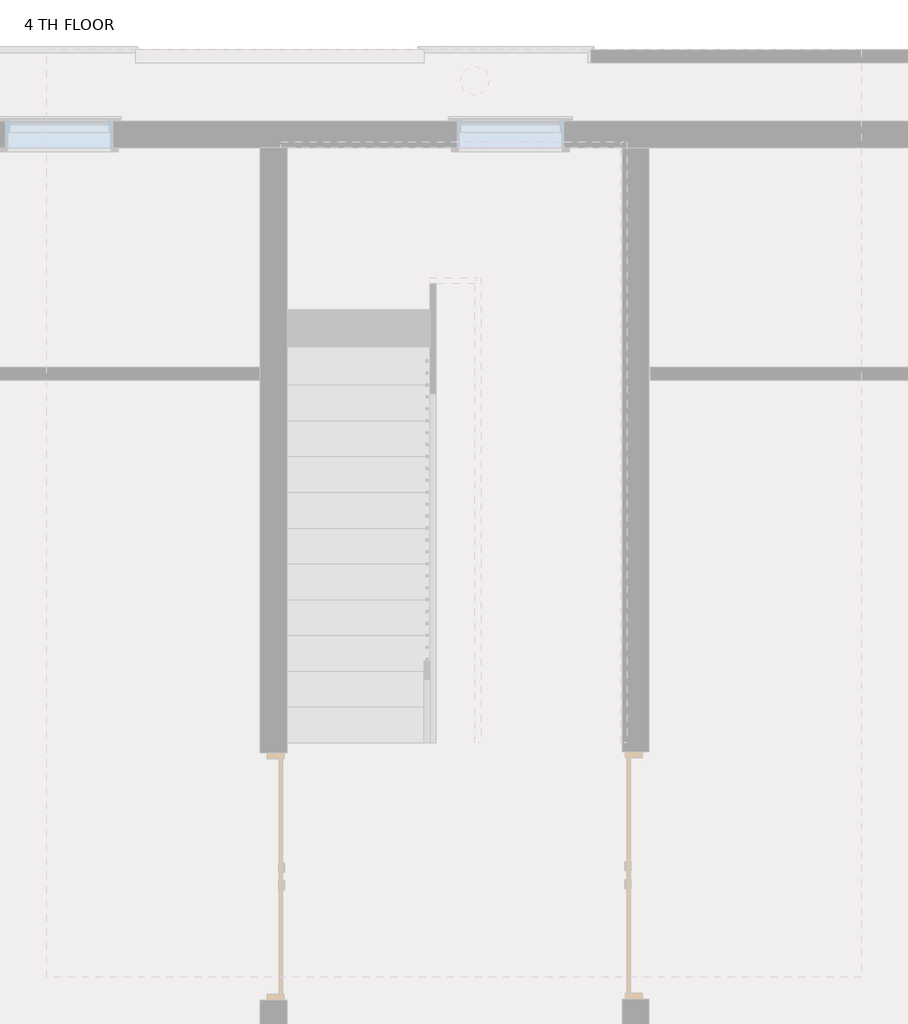
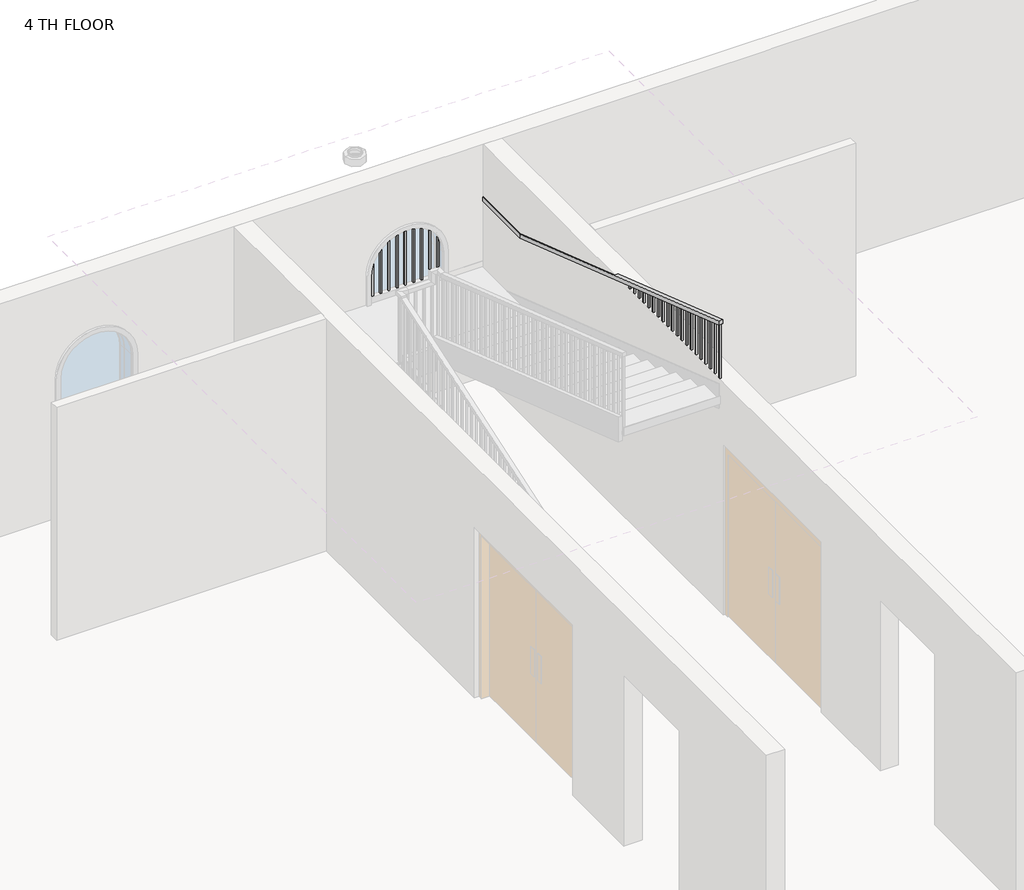
# One storey, part 5 of 7: 1 railing.
"""IFC4 building model written with IfcOpenShell, lengths in millimetres."""

from ifc_helpers import new_model, si_unit, frame, origin, place, context, project, spatial, polyline, outline, extrude, faceted_brep, element, save

model = new_model("IFC4")

# Units and contexts
model_context = context("Model", 3, world=origin())
ifc_project = project(units=[si_unit("LENGTHUNIT", "METRE", prefix="MILLI")], contexts=[model_context])

# Site, building, storey
site = spatial("IfcSite", under=ifc_project)
building = spatial("IfcBuilding", under=site)
storey = spatial("IfcBuildingStorey", under=building, Name="4 TH FLOOR", Elevation=12801.6)

# Railing
placement = place(None, origin())
element("IfcRailing", 1, ObjectType="Handrail - Rectangular", at=placement, inside=storey, context=model_context, shape_type="SolidModel", body=[
    faceted_brep([(-1899.5987998, 2564.5067329, 13819.4142857), (-1899.5987998, 2564.5067329, 13765.7699957), (-1848.7987998, 2564.5067329, 13765.7699957), (-1848.7987998, 2564.5067329, 13819.4142857), (-1899.5987998, 6526.9067329, 15163.8), (-1899.5987998, 6535.2899033, 15113.0), (-1848.7987998, 6535.2899033, 15113.0), (-1848.7987998, 6526.9067329, 15163.8), (-1899.5987998, 7682.6067329, 15113.0), (-1899.5987998, 7682.6067329, 15163.8), (1046.8012002, 7682.6067329, 15163.8), (1046.8012002, 7682.6067329, 15113.0), (-1848.7987998, 7631.8067329, 15113.0), (996.0012002, 7631.8067329, 15113.0), (-1848.7987998, 7631.8067329, 15163.8), (996.0012002, 7631.8067329, 15163.8), (1046.8012002, 6831.7067329, 15163.8), (1046.8012002, 6823.3235624, 15113.0), (996.0012002, 6823.3235624, 15113.0), (996.0012002, 6831.7067329, 15163.8), (1046.8012002, 2564.5067329, 16611.6), (996.0012002, 2564.5067329, 16611.6), (996.0012002, 2564.5067329, 16557.95571), (1046.8012002, 2564.5067329, 16557.95571)], [[[0, 1, 2, 3]], [[1, 0, 4, 5]], [[2, 1, 5, 6]], [[3, 2, 6, 7]], [[0, 3, 7, 4]], [[8, 9, 10, 11]], [[12, 8, 11, 13]], [[14, 12, 13, 15]], [[9, 14, 15, 10]], [[11, 10, 16, 17]], [[13, 11, 17, 18]], [[15, 13, 18, 19]], [[10, 15, 19, 16]], [[5, 4, 9, 8]], [[6, 5, 8, 12]], [[7, 6, 12, 14]], [[4, 7, 14, 9]], [[20, 21, 22, 23]], [[17, 16, 20, 23]], [[18, 17, 23, 22]], [[19, 18, 22, 21]], [[16, 19, 21, 20]]]),
    extrude(outline(polyline([(2586.7317329, 16550.415085), (2586.7317329, 15779.4831452), (2567.6817329, 15785.9465381), (2567.6817329, 16556.8784779), (2586.7317329, 16550.415085)])), frame((1011.8762002, 0.0, 0.0), z_axis=(1.0, 0.0, 0.0), x_axis=(0.0, 1.0, 0.0)), (0.0, 0.0, 1.0), 19.05),
    extrude(outline(polyline([(2688.3317329, 16515.9436565), (2688.3317329, 15745.0117167), (2669.2817329, 15751.4751095), (2669.2817329, 16522.4070493), (2688.3317329, 16515.9436565)])), frame((1011.8762002, 0.0, 0.0), z_axis=(1.0, 0.0, 0.0), x_axis=(0.0, 1.0, 0.0)), (0.0, 0.0, 1.0), 19.05),
    extrude(outline(polyline([(2789.9317329, 16481.4722279), (2789.9317329, 15710.5402881), (2770.8817329, 15717.003681), (2770.8817329, 16487.9356207), (2789.9317329, 16481.4722279)])), frame((1011.8762002, 0.0, 0.0), z_axis=(1.0, 0.0, 0.0), x_axis=(0.0, 1.0, 0.0)), (0.0, 0.0, 1.0), 19.05),
    extrude(outline(polyline([(2891.5317329, 16447.0007993), (2891.5317329, 15676.0688595), (2872.4817329, 15682.5322524), (2872.4817329, 16453.4641922), (2891.5317329, 16447.0007993)])), frame((1011.8762002, 0.0, 0.0), z_axis=(1.0, 0.0, 0.0), x_axis=(0.0, 1.0, 0.0)), (0.0, 0.0, 1.0), 19.05),
    extrude(outline(polyline([(2993.1317329, 16412.5293707), (2993.1317329, 15641.597431), (2974.0817329, 15648.0608238), (2974.0817329, 16418.9927636), (2993.1317329, 16412.5293707)])), frame((1011.8762002, 0.0, 0.0), z_axis=(1.0, 0.0, 0.0), x_axis=(0.0, 1.0, 0.0)), (0.0, 0.0, 1.0), 19.05),
    extrude(outline(polyline([(3094.7317329, 16378.0579422), (3094.7317329, 15607.1260024), (3075.6817329, 15613.5893952), (3075.6817329, 16384.521335), (3094.7317329, 16378.0579422)])), frame((1011.8762002, 0.0, 0.0), z_axis=(1.0, 0.0, 0.0), x_axis=(0.0, 1.0, 0.0)), (0.0, 0.0, 1.0), 19.05),
    extrude(outline(polyline([(3196.3317329, 16343.5865136), (3196.3317329, 15572.6545738), (3177.2817329, 15579.1179667), (3177.2817329, 16350.0499065), (3196.3317329, 16343.5865136)])), frame((1011.8762002, 0.0, 0.0), z_axis=(1.0, 0.0, 0.0), x_axis=(0.0, 1.0, 0.0)), (0.0, 0.0, 1.0), 19.05),
    extrude(outline(polyline([(3297.9317329, 16309.115085), (3297.9317329, 15538.1831452), (3278.8817329, 15544.6465381), (3278.8817329, 16315.5784779), (3297.9317329, 16309.115085)])), frame((1011.8762002, 0.0, 0.0), z_axis=(1.0, 0.0, 0.0), x_axis=(0.0, 1.0, 0.0)), (0.0, 0.0, 1.0), 19.05),
    extrude(outline(polyline([(3399.5317329, 16274.6436565), (3399.5317329, 15503.7117167), (3380.4817329, 15510.1751095), (3380.4817329, 16281.1070493), (3399.5317329, 16274.6436565)])), frame((1011.8762002, 0.0, 0.0), z_axis=(1.0, 0.0, 0.0), x_axis=(0.0, 1.0, 0.0)), (0.0, 0.0, 1.0), 19.05),
    extrude(outline(polyline([(3501.1317329, 16240.1722279), (3501.1317329, 15469.2402881), (3482.0817329, 15475.703681), (3482.0817329, 16246.6356207), (3501.1317329, 16240.1722279)])), frame((1011.8762002, 0.0, 0.0), z_axis=(1.0, 0.0, 0.0), x_axis=(0.0, 1.0, 0.0)), (0.0, 0.0, 1.0), 19.05),
    extrude(outline(polyline([(3602.7317329, 16205.7007993), (3602.7317329, 15434.7688595), (3583.6817329, 15441.2322524), (3583.6817329, 16212.1641922), (3602.7317329, 16205.7007993)])), frame((1011.8762002, 0.0, 0.0), z_axis=(1.0, 0.0, 0.0), x_axis=(0.0, 1.0, 0.0)), (0.0, 0.0, 1.0), 19.05),
    extrude(outline(polyline([(3704.3317329, 16171.2293707), (3704.3317329, 15400.297431), (3685.2817329, 15406.7608238), (3685.2817329, 16177.6927636), (3704.3317329, 16171.2293707)])), frame((1011.8762002, 0.0, 0.0), z_axis=(1.0, 0.0, 0.0), x_axis=(0.0, 1.0, 0.0)), (0.0, 0.0, 1.0), 19.05),
    extrude(outline(polyline([(3805.9317329, 16136.7579422), (3805.9317329, 15365.8260024), (3786.8817329, 15372.2893952), (3786.8817329, 16143.221335), (3805.9317329, 16136.7579422)])), frame((1011.8762002, 0.0, 0.0), z_axis=(1.0, 0.0, 0.0), x_axis=(0.0, 1.0, 0.0)), (0.0, 0.0, 1.0), 19.05),
    extrude(outline(polyline([(3907.5317329, 16102.2865136), (3907.5317329, 15331.3545738), (3888.4817329, 15337.8179667), (3888.4817329, 16108.7499065), (3907.5317329, 16102.2865136)])), frame((1011.8762002, 0.0, 0.0), z_axis=(1.0, 0.0, 0.0), x_axis=(0.0, 1.0, 0.0)), (0.0, 0.0, 1.0), 19.05),
    extrude(outline(polyline([(4009.1317329, 16067.815085), (4009.1317329, 15296.8831452), (3990.0817329, 15303.3465381), (3990.0817329, 16074.2784779), (4009.1317329, 16067.815085)])), frame((1011.8762002, 0.0, 0.0), z_axis=(1.0, 0.0, 0.0), x_axis=(0.0, 1.0, 0.0)), (0.0, 0.0, 1.0), 19.05),
    extrude(outline(polyline([(4110.7317329, 16033.3436565), (4110.7317329, 15262.4117167), (4091.6817329, 15268.8751095), (4091.6817329, 16039.8070493), (4110.7317329, 16033.3436565)])), frame((1011.8762002, 0.0, 0.0), z_axis=(1.0, 0.0, 0.0), x_axis=(0.0, 1.0, 0.0)), (0.0, 0.0, 1.0), 19.05),
    extrude(outline(polyline([(4212.3317329, 15998.8722279), (4212.3317329, 15227.9402881), (4193.2817329, 15234.403681), (4193.2817329, 16005.3356207), (4212.3317329, 15998.8722279)])), frame((1011.8762002, 0.0, 0.0), z_axis=(1.0, 0.0, 0.0), x_axis=(0.0, 1.0, 0.0)), (0.0, 0.0, 1.0), 19.05),
    extrude(outline(polyline([(4313.9317329, 15964.4007993), (4313.9317329, 15193.4688595), (4294.8817329, 15199.9322524), (4294.8817329, 15970.8641922), (4313.9317329, 15964.4007993)])), frame((1011.8762002, 0.0, 0.0), z_axis=(1.0, 0.0, 0.0), x_axis=(0.0, 1.0, 0.0)), (0.0, 0.0, 1.0), 19.05),
    extrude(outline(polyline([(4415.5317329, 15929.9293707), (4415.5317329, 15158.997431), (4396.4817329, 15165.4608238), (4396.4817329, 15936.3927636), (4415.5317329, 15929.9293707)])), frame((1011.8762002, 0.0, 0.0), z_axis=(1.0, 0.0, 0.0), x_axis=(0.0, 1.0, 0.0)), (0.0, 0.0, 1.0), 19.05),
    extrude(outline(polyline([(4517.1317329, 15895.4579422), (4517.1317329, 15124.5260024), (4498.0817329, 15130.9893952), (4498.0817329, 15901.921335), (4517.1317329, 15895.4579422)])), frame((1011.8762002, 0.0, 0.0), z_axis=(1.0, 0.0, 0.0), x_axis=(0.0, 1.0, 0.0)), (0.0, 0.0, 1.0), 19.05),
    extrude(outline(polyline([(4618.7317329, 15860.9865136), (4618.7317329, 15090.0545738), (4599.6817329, 15096.5179667), (4599.6817329, 15867.4499065), (4618.7317329, 15860.9865136)])), frame((1011.8762002, 0.0, 0.0), z_axis=(1.0, 0.0, 0.0), x_axis=(0.0, 1.0, 0.0)), (0.0, 0.0, 1.0), 19.05),
    extrude(outline(polyline([(4720.3317329, 15826.515085), (4720.3317329, 15055.5831452), (4701.2817329, 15062.0465381), (4701.2817329, 15832.9784779), (4720.3317329, 15826.515085)])), frame((1011.8762002, 0.0, 0.0), z_axis=(1.0, 0.0, 0.0), x_axis=(0.0, 1.0, 0.0)), (0.0, 0.0, 1.0), 19.05),
    extrude(outline(polyline([(4821.9317329, 15792.0436565), (4821.9317329, 15021.1117167), (4802.8817329, 15027.5751095), (4802.8817329, 15798.5070493), (4821.9317329, 15792.0436565)])), frame((1011.8762002, 0.0, 0.0), z_axis=(1.0, 0.0, 0.0), x_axis=(0.0, 1.0, 0.0)), (0.0, 0.0, 1.0), 19.05),
    extrude(outline(polyline([(4923.5317329, 15757.5722279), (4923.5317329, 14986.6402881), (4904.4817329, 14993.103681), (4904.4817329, 15764.0356207), (4923.5317329, 15757.5722279)])), frame((1011.8762002, 0.0, 0.0), z_axis=(1.0, 0.0, 0.0), x_axis=(0.0, 1.0, 0.0)), (0.0, 0.0, 1.0), 19.05),
    extrude(outline(polyline([(5025.1317329, 15723.1007993), (5025.1317329, 14952.1688595), (5006.0817329, 14958.6322524), (5006.0817329, 15729.5641922), (5025.1317329, 15723.1007993)])), frame((1011.8762002, 0.0, 0.0), z_axis=(1.0, 0.0, 0.0), x_axis=(0.0, 1.0, 0.0)), (0.0, 0.0, 1.0), 19.05),
    extrude(outline(polyline([(5126.7317329, 15688.6293707), (5126.7317329, 14917.697431), (5107.6817329, 14924.1608238), (5107.6817329, 15695.0927636), (5126.7317329, 15688.6293707)])), frame((1011.8762002, 0.0, 0.0), z_axis=(1.0, 0.0, 0.0), x_axis=(0.0, 1.0, 0.0)), (0.0, 0.0, 1.0), 19.05),
    extrude(outline(polyline([(5228.3317329, 15654.1579422), (5228.3317329, 14883.2260024), (5209.2817329, 14889.6893952), (5209.2817329, 15660.621335), (5228.3317329, 15654.1579422)])), frame((1011.8762002, 0.0, 0.0), z_axis=(1.0, 0.0, 0.0), x_axis=(0.0, 1.0, 0.0)), (0.0, 0.0, 1.0), 19.05),
    extrude(outline(polyline([(5329.9317329, 15619.6865136), (5329.9317329, 14848.7545738), (5310.8817329, 14855.2179667), (5310.8817329, 15626.1499065), (5329.9317329, 15619.6865136)])), frame((1011.8762002, 0.0, 0.0), z_axis=(1.0, 0.0, 0.0), x_axis=(0.0, 1.0, 0.0)), (0.0, 0.0, 1.0), 19.05),
    extrude(outline(polyline([(5431.5317329, 15585.215085), (5431.5317329, 14814.2831452), (5412.4817329, 14820.7465381), (5412.4817329, 15591.6784779), (5431.5317329, 15585.215085)])), frame((1011.8762002, 0.0, 0.0), z_axis=(1.0, 0.0, 0.0), x_axis=(0.0, 1.0, 0.0)), (0.0, 0.0, 1.0), 19.05),
    extrude(outline(polyline([(5533.1317329, 15550.7436565), (5533.1317329, 14779.8117167), (5514.0817329, 14786.2751095), (5514.0817329, 15557.2070493), (5533.1317329, 15550.7436565)])), frame((1011.8762002, 0.0, 0.0), z_axis=(1.0, 0.0, 0.0), x_axis=(0.0, 1.0, 0.0)), (0.0, 0.0, 1.0), 19.05),
    extrude(outline(polyline([(5634.7317329, 15516.2722279), (5634.7317329, 14745.3402881), (5615.6817329, 14751.803681), (5615.6817329, 15522.7356207), (5634.7317329, 15516.2722279)])), frame((1011.8762002, 0.0, 0.0), z_axis=(1.0, 0.0, 0.0), x_axis=(0.0, 1.0, 0.0)), (0.0, 0.0, 1.0), 19.05),
    extrude(outline(polyline([(5736.3317329, 15481.8007993), (5736.3317329, 14710.8688595), (5717.2817329, 14717.3322524), (5717.2817329, 15488.2641922), (5736.3317329, 15481.8007993)])), frame((1011.8762002, 0.0, 0.0), z_axis=(1.0, 0.0, 0.0), x_axis=(0.0, 1.0, 0.0)), (0.0, 0.0, 1.0), 19.05),
    extrude(outline(polyline([(5837.9317329, 15447.3293707), (5837.9317329, 14676.397431), (5818.8817329, 14682.8608238), (5818.8817329, 15453.7927636), (5837.9317329, 15447.3293707)])), frame((1011.8762002, 0.0, 0.0), z_axis=(1.0, 0.0, 0.0), x_axis=(0.0, 1.0, 0.0)), (0.0, 0.0, 1.0), 19.05),
    extrude(outline(polyline([(5939.5317329, 15412.8579422), (5939.5317329, 14641.9260024), (5920.4817329, 14648.3893952), (5920.4817329, 15419.321335), (5939.5317329, 15412.8579422)])), frame((1011.8762002, 0.0, 0.0), z_axis=(1.0, 0.0, 0.0), x_axis=(0.0, 1.0, 0.0)), (0.0, 0.0, 1.0), 19.05),
    extrude(outline(polyline([(6041.1317329, 15378.3865136), (6041.1317329, 14607.4545738), (6022.0817329, 14613.9179667), (6022.0817329, 15384.8499065), (6041.1317329, 15378.3865136)])), frame((1011.8762002, 0.0, 0.0), z_axis=(1.0, 0.0, 0.0), x_axis=(0.0, 1.0, 0.0)), (0.0, 0.0, 1.0), 19.05),
    extrude(outline(polyline([(6142.7317329, 15343.915085), (6142.7317329, 14572.9831452), (6123.6817329, 14579.4465381), (6123.6817329, 15350.3784779), (6142.7317329, 15343.915085)])), frame((1011.8762002, 0.0, 0.0), z_axis=(1.0, 0.0, 0.0), x_axis=(0.0, 1.0, 0.0)), (0.0, 0.0, 1.0), 19.05),
    extrude(outline(polyline([(6244.3317329, 15309.4436565), (6244.3317329, 14538.5117167), (6225.2817329, 14544.9751095), (6225.2817329, 15315.9070493), (6244.3317329, 15309.4436565)])), frame((1011.8762002, 0.0, 0.0), z_axis=(1.0, 0.0, 0.0), x_axis=(0.0, 1.0, 0.0)), (0.0, 0.0, 1.0), 19.05),
    extrude(outline(polyline([(6345.9317329, 15274.9722279), (6345.9317329, 14504.0402881), (6326.8817329, 14510.503681), (6326.8817329, 15281.4356207), (6345.9317329, 15274.9722279)])), frame((1011.8762002, 0.0, 0.0), z_axis=(1.0, 0.0, 0.0), x_axis=(0.0, 1.0, 0.0)), (0.0, 0.0, 1.0), 19.05),
    extrude(outline(polyline([(6447.5317329, 15240.5007993), (6447.5317329, 14469.5688595), (6428.4817329, 14476.0322524), (6428.4817329, 15246.9641922), (6447.5317329, 15240.5007993)])), frame((1011.8762002, 0.0, 0.0), z_axis=(1.0, 0.0, 0.0), x_axis=(0.0, 1.0, 0.0)), (0.0, 0.0, 1.0), 19.05),
    extrude(outline(polyline([(6549.1317329, 15206.0293707), (6549.1317329, 14435.097431), (6530.0817329, 14441.5608238), (6530.0817329, 15212.4927636), (6549.1317329, 15206.0293707)])), frame((1011.8762002, 0.0, 0.0), z_axis=(1.0, 0.0, 0.0), x_axis=(0.0, 1.0, 0.0)), (0.0, 0.0, 1.0), 19.05),
    extrude(outline(polyline([(6650.7317329, 15171.5579422), (6650.7317329, 14400.6260024), (6631.6817329, 14407.0893952), (6631.6817329, 15178.021335), (6650.7317329, 15171.5579422)])), frame((1011.8762002, 0.0, 0.0), z_axis=(1.0, 0.0, 0.0), x_axis=(0.0, 1.0, 0.0)), (0.0, 0.0, 1.0), 19.05),
    extrude(outline(polyline([(6752.3317329, 15137.0865136), (6752.3317329, 14366.1545738), (6733.2817329, 14372.6179667), (6733.2817329, 15143.5499065), (6752.3317329, 15137.0865136)])), frame((1011.8762002, 0.0, 0.0), z_axis=(1.0, 0.0, 0.0), x_axis=(0.0, 1.0, 0.0)), (0.0, 0.0, 1.0), 19.05),
    extrude(outline(polyline([(6853.9317329, 15113.0), (6853.9317329, 14331.6831452), (6834.8817329, 14338.1465381), (6834.8817329, 15113.0), (6853.9317329, 15113.0)])), frame((1011.8762002, 0.0, 0.0), z_axis=(1.0, 0.0, 0.0), x_axis=(0.0, 1.0, 0.0)), (0.0, 0.0, 1.0), 19.05),
    extrude(outline(polyline([(6955.5317329, 15113.0), (6955.5317329, 14297.2117167), (6936.4817329, 14303.6751095), (6936.4817329, 15113.0), (6955.5317329, 15113.0)])), frame((1011.8762002, 0.0, 0.0), z_axis=(1.0, 0.0, 0.0), x_axis=(0.0, 1.0, 0.0)), (0.0, 0.0, 1.0), 19.05),
    extrude(outline(polyline([(7057.1317329, 15113.0), (7057.1317329, 14262.7402881), (7038.0817329, 14269.203681), (7038.0817329, 15113.0), (7057.1317329, 15113.0)])), frame((1011.8762002, 0.0, 0.0), z_axis=(1.0, 0.0, 0.0), x_axis=(0.0, 1.0, 0.0)), (0.0, 0.0, 1.0), 19.05),
    extrude(outline(polyline([(7158.7317329, 15113.0), (7158.7317329, 14228.2688595), (7139.6817329, 14234.7322524), (7139.6817329, 15113.0), (7158.7317329, 15113.0)])), frame((1011.8762002, 0.0, 0.0), z_axis=(1.0, 0.0, 0.0), x_axis=(0.0, 1.0, 0.0)), (0.0, 0.0, 1.0), 19.05),
    extrude(outline(polyline([(7260.3317329, 15113.0), (7260.3317329, 14193.797431), (7241.2817329, 14200.2608238), (7241.2817329, 15113.0), (7260.3317329, 15113.0)])), frame((1011.8762002, 0.0, 0.0), z_axis=(1.0, 0.0, 0.0), x_axis=(0.0, 1.0, 0.0)), (0.0, 0.0, 1.0), 19.05),
    extrude(outline(polyline([(7361.9317329, 15113.0), (7361.9317329, 14159.3260024), (7342.8817329, 14165.7893952), (7342.8817329, 15113.0), (7361.9317329, 15113.0)])), frame((1011.8762002, 0.0, 0.0), z_axis=(1.0, 0.0, 0.0), x_axis=(0.0, 1.0, 0.0)), (0.0, 0.0, 1.0), 19.05),
    extrude(outline(polyline([(7463.5317329, 15113.0), (7463.5317329, 14124.8545738), (7444.4817329, 14131.3179667), (7444.4817329, 15113.0), (7463.5317329, 15113.0)])), frame((1011.8762002, 0.0, 0.0), z_axis=(1.0, 0.0, 0.0), x_axis=(0.0, 1.0, 0.0)), (0.0, 0.0, 1.0), 19.05),
    extrude(outline(polyline([(7565.1317329, 15113.0), (7565.1317329, 14090.3831452), (7546.0817329, 14096.8465381), (7546.0817329, 15113.0), (7565.1317329, 15113.0)])), frame((1011.8762002, 0.0, 0.0), z_axis=(1.0, 0.0, 0.0), x_axis=(0.0, 1.0, 0.0)), (0.0, 0.0, 1.0), 19.05),
    extrude(outline(polyline([(961.0762002, 7666.7317329), (980.1262002, 7666.7317329), (980.1262002, 7647.6817329), (961.0762002, 7647.6817329), (961.0762002, 7666.7317329)])), frame((0.0, 0.0, 14325.6), z_axis=(0.0, 0.0, 1.0), x_axis=(1.0, 0.0, 0.0)), (0.0, 0.0, 1.0), 787.4),
    extrude(outline(polyline([(859.4762002, 7666.7317329), (878.5262002, 7666.7317329), (878.5262002, 7647.6817329), (859.4762002, 7647.6817329), (859.4762002, 7666.7317329)])), frame((0.0, 0.0, 14325.6), z_axis=(0.0, 0.0, 1.0), x_axis=(1.0, 0.0, 0.0)), (0.0, 0.0, 1.0), 787.4),
    extrude(outline(polyline([(757.8762002, 7666.7317329), (776.9262002, 7666.7317329), (776.9262002, 7647.6817329), (757.8762002, 7647.6817329), (757.8762002, 7666.7317329)])), frame((0.0, 0.0, 14325.6), z_axis=(0.0, 0.0, 1.0), x_axis=(1.0, 0.0, 0.0)), (0.0, 0.0, 1.0), 787.4),
    extrude(outline(polyline([(656.2762002, 7666.7317329), (675.3262002, 7666.7317329), (675.3262002, 7647.6817329), (656.2762002, 7647.6817329), (656.2762002, 7666.7317329)])), frame((0.0, 0.0, 14325.6), z_axis=(0.0, 0.0, 1.0), x_axis=(1.0, 0.0, 0.0)), (0.0, 0.0, 1.0), 787.4),
    extrude(outline(polyline([(554.6762002, 7666.7317329), (573.7262002, 7666.7317329), (573.7262002, 7647.6817329), (554.6762002, 7647.6817329), (554.6762002, 7666.7317329)])), frame((0.0, 0.0, 14325.6), z_axis=(0.0, 0.0, 1.0), x_axis=(1.0, 0.0, 0.0)), (0.0, 0.0, 1.0), 787.4),
    extrude(outline(polyline([(453.0762002, 7666.7317329), (472.1262002, 7666.7317329), (472.1262002, 7647.6817329), (453.0762002, 7647.6817329), (453.0762002, 7666.7317329)])), frame((0.0, 0.0, 14325.6), z_axis=(0.0, 0.0, 1.0), x_axis=(1.0, 0.0, 0.0)), (0.0, 0.0, 1.0), 787.4),
    extrude(outline(polyline([(351.4762002, 7666.7317329), (370.5262002, 7666.7317329), (370.5262002, 7647.6817329), (351.4762002, 7647.6817329), (351.4762002, 7666.7317329)])), frame((0.0, 0.0, 14325.6), z_axis=(0.0, 0.0, 1.0), x_axis=(1.0, 0.0, 0.0)), (0.0, 0.0, 1.0), 787.4),
    extrude(outline(polyline([(249.8762002, 7666.7317329), (268.9262002, 7666.7317329), (268.9262002, 7647.6817329), (249.8762002, 7647.6817329), (249.8762002, 7666.7317329)])), frame((0.0, 0.0, 14325.6), z_axis=(0.0, 0.0, 1.0), x_axis=(1.0, 0.0, 0.0)), (0.0, 0.0, 1.0), 787.4),
    extrude(outline(polyline([(148.2762002, 7666.7317329), (167.3262002, 7666.7317329), (167.3262002, 7647.6817329), (148.2762002, 7647.6817329), (148.2762002, 7666.7317329)])), frame((0.0, 0.0, 14325.6), z_axis=(0.0, 0.0, 1.0), x_axis=(1.0, 0.0, 0.0)), (0.0, 0.0, 1.0), 787.4),
    extrude(outline(polyline([(46.6762002, 7666.7317329), (65.7262002, 7666.7317329), (65.7262002, 7647.6817329), (46.6762002, 7647.6817329), (46.6762002, 7666.7317329)])), frame((0.0, 0.0, 14325.6), z_axis=(0.0, 0.0, 1.0), x_axis=(1.0, 0.0, 0.0)), (0.0, 0.0, 1.0), 787.4),
    extrude(outline(polyline([(-54.9237998, 7666.7317329), (-35.8737998, 7666.7317329), (-35.8737998, 7647.6817329), (-54.9237998, 7647.6817329), (-54.9237998, 7666.7317329)])), frame((0.0, 0.0, 14325.6), z_axis=(0.0, 0.0, 1.0), x_axis=(1.0, 0.0, 0.0)), (0.0, 0.0, 1.0), 787.4),
    extrude(outline(polyline([(-156.5237998, 7666.7317329), (-137.4737998, 7666.7317329), (-137.4737998, 7647.6817329), (-156.5237998, 7647.6817329), (-156.5237998, 7666.7317329)])), frame((0.0, 0.0, 14325.6), z_axis=(0.0, 0.0, 1.0), x_axis=(1.0, 0.0, 0.0)), (0.0, 0.0, 1.0), 787.4),
    extrude(outline(polyline([(-258.1237998, 7666.7317329), (-239.0737998, 7666.7317329), (-239.0737998, 7647.6817329), (-258.1237998, 7647.6817329), (-258.1237998, 7666.7317329)])), frame((0.0, 0.0, 14325.6), z_axis=(0.0, 0.0, 1.0), x_axis=(1.0, 0.0, 0.0)), (0.0, 0.0, 1.0), 787.4),
    extrude(outline(polyline([(-359.7237998, 7666.7317329), (-340.6737998, 7666.7317329), (-340.6737998, 7647.6817329), (-359.7237998, 7647.6817329), (-359.7237998, 7666.7317329)])), frame((0.0, 0.0, 14325.6), z_axis=(0.0, 0.0, 1.0), x_axis=(1.0, 0.0, 0.0)), (0.0, 0.0, 1.0), 787.4),
    extrude(outline(polyline([(-461.3237998, 7666.7317329), (-442.2737998, 7666.7317329), (-442.2737998, 7647.6817329), (-461.3237998, 7647.6817329), (-461.3237998, 7666.7317329)])), frame((0.0, 0.0, 14325.6), z_axis=(0.0, 0.0, 1.0), x_axis=(1.0, 0.0, 0.0)), (0.0, 0.0, 1.0), 787.4),
    extrude(outline(polyline([(-562.9237998, 7666.7317329), (-543.8737998, 7666.7317329), (-543.8737998, 7647.6817329), (-562.9237998, 7647.6817329), (-562.9237998, 7666.7317329)])), frame((0.0, 0.0, 14325.6), z_axis=(0.0, 0.0, 1.0), x_axis=(1.0, 0.0, 0.0)), (0.0, 0.0, 1.0), 787.4),
    extrude(outline(polyline([(-664.5237998, 7666.7317329), (-645.4737998, 7666.7317329), (-645.4737998, 7647.6817329), (-664.5237998, 7647.6817329), (-664.5237998, 7666.7317329)])), frame((0.0, 0.0, 14325.6), z_axis=(0.0, 0.0, 1.0), x_axis=(1.0, 0.0, 0.0)), (0.0, 0.0, 1.0), 787.4),
    extrude(outline(polyline([(-766.1237998, 7666.7317329), (-747.0737998, 7666.7317329), (-747.0737998, 7647.6817329), (-766.1237998, 7647.6817329), (-766.1237998, 7666.7317329)])), frame((0.0, 0.0, 14325.6), z_axis=(0.0, 0.0, 1.0), x_axis=(1.0, 0.0, 0.0)), (0.0, 0.0, 1.0), 787.4),
    extrude(outline(polyline([(-867.7237998, 7666.7317329), (-848.6737998, 7666.7317329), (-848.6737998, 7647.6817329), (-867.7237998, 7647.6817329), (-867.7237998, 7666.7317329)])), frame((0.0, 0.0, 14325.6), z_axis=(0.0, 0.0, 1.0), x_axis=(1.0, 0.0, 0.0)), (0.0, 0.0, 1.0), 787.4),
    extrude(outline(polyline([(-969.3237998, 7666.7317329), (-950.2737998, 7666.7317329), (-950.2737998, 7647.6817329), (-969.3237998, 7647.6817329), (-969.3237998, 7666.7317329)])), frame((0.0, 0.0, 14325.6), z_axis=(0.0, 0.0, 1.0), x_axis=(1.0, 0.0, 0.0)), (0.0, 0.0, 1.0), 787.4),
    extrude(outline(polyline([(-1070.9237998, 7666.7317329), (-1051.8737998, 7666.7317329), (-1051.8737998, 7647.6817329), (-1070.9237998, 7647.6817329), (-1070.9237998, 7666.7317329)])), frame((0.0, 0.0, 14325.6), z_axis=(0.0, 0.0, 1.0), x_axis=(1.0, 0.0, 0.0)), (0.0, 0.0, 1.0), 787.4),
    extrude(outline(polyline([(-1172.5237998, 7666.7317329), (-1153.4737998, 7666.7317329), (-1153.4737998, 7647.6817329), (-1172.5237998, 7647.6817329), (-1172.5237998, 7666.7317329)])), frame((0.0, 0.0, 14325.6), z_axis=(0.0, 0.0, 1.0), x_axis=(1.0, 0.0, 0.0)), (0.0, 0.0, 1.0), 787.4),
    extrude(outline(polyline([(-1274.1237998, 7666.7317329), (-1255.0737998, 7666.7317329), (-1255.0737998, 7647.6817329), (-1274.1237998, 7647.6817329), (-1274.1237998, 7666.7317329)])), frame((0.0, 0.0, 14325.6), z_axis=(0.0, 0.0, 1.0), x_axis=(1.0, 0.0, 0.0)), (0.0, 0.0, 1.0), 787.4),
    extrude(outline(polyline([(-1375.7237998, 7666.7317329), (-1356.6737998, 7666.7317329), (-1356.6737998, 7647.6817329), (-1375.7237998, 7647.6817329), (-1375.7237998, 7666.7317329)])), frame((0.0, 0.0, 14325.6), z_axis=(0.0, 0.0, 1.0), x_axis=(1.0, 0.0, 0.0)), (0.0, 0.0, 1.0), 787.4),
    extrude(outline(polyline([(-1477.3237998, 7666.7317329), (-1458.2737998, 7666.7317329), (-1458.2737998, 7647.6817329), (-1477.3237998, 7647.6817329), (-1477.3237998, 7666.7317329)])), frame((0.0, 0.0, 14325.6), z_axis=(0.0, 0.0, 1.0), x_axis=(1.0, 0.0, 0.0)), (0.0, 0.0, 1.0), 787.4),
    extrude(outline(polyline([(-1578.9237998, 7666.7317329), (-1559.8737998, 7666.7317329), (-1559.8737998, 7647.6817329), (-1578.9237998, 7647.6817329), (-1578.9237998, 7666.7317329)])), frame((0.0, 0.0, 14325.6), z_axis=(0.0, 0.0, 1.0), x_axis=(1.0, 0.0, 0.0)), (0.0, 0.0, 1.0), 787.4),
    extrude(outline(polyline([(-1680.5237998, 7666.7317329), (-1661.4737998, 7666.7317329), (-1661.4737998, 7647.6817329), (-1680.5237998, 7647.6817329), (-1680.5237998, 7666.7317329)])), frame((0.0, 0.0, 14325.6), z_axis=(0.0, 0.0, 1.0), x_axis=(1.0, 0.0, 0.0)), (0.0, 0.0, 1.0), 787.4),
    extrude(outline(polyline([(-1782.1237998, 7666.7317329), (-1763.0737998, 7666.7317329), (-1763.0737998, 7647.6817329), (-1782.1237998, 7647.6817329), (-1782.1237998, 7666.7317329)])), frame((0.0, 0.0, 14325.6), z_axis=(0.0, 0.0, 1.0), x_axis=(1.0, 0.0, 0.0)), (0.0, 0.0, 1.0), 787.4),
    extrude(outline(polyline([(-1883.7237998, 7634.9817329), (-1883.7237998, 7654.0317329), (-1864.6737998, 7654.0317329), (-1864.6737998, 7634.9817329), (-1883.7237998, 7634.9817329)])), frame((0.0, 0.0, 14628.5857143), z_axis=(0.0, 0.0, 1.0), x_axis=(1.0, 0.0, 0.0)), (0.0, 0.0, 1.0), 484.4142857),
    extrude(outline(polyline([(-1883.7237998, 7533.3817329), (-1883.7237998, 7552.4317329), (-1864.6737998, 7552.4317329), (-1864.6737998, 7533.3817329), (-1883.7237998, 7533.3817329)])), frame((0.0, 0.0, 14594.1142857), z_axis=(0.0, 0.0, 1.0), x_axis=(1.0, 0.0, 0.0)), (0.0, 0.0, 1.0), 518.8857143),
    extrude(outline(polyline([(-1883.7237998, 7431.7817329), (-1883.7237998, 7450.8317329), (-1864.6737998, 7450.8317329), (-1864.6737998, 7431.7817329), (-1883.7237998, 7431.7817329)])), frame((0.0, 0.0, 14559.6428571), z_axis=(0.0, 0.0, 1.0), x_axis=(1.0, 0.0, 0.0)), (0.0, 0.0, 1.0), 553.3571429),
    extrude(outline(polyline([(-1883.7237998, 7330.1817329), (-1883.7237998, 7349.2317329), (-1864.6737998, 7349.2317329), (-1864.6737998, 7330.1817329), (-1883.7237998, 7330.1817329)])), frame((0.0, 0.0, 14525.1714286), z_axis=(0.0, 0.0, 1.0), x_axis=(1.0, 0.0, 0.0)), (0.0, 0.0, 1.0), 587.8285714),
    extrude(outline(polyline([(-1883.7237998, 7228.5817329), (-1883.7237998, 7247.6317329), (-1864.6737998, 7247.6317329), (-1864.6737998, 7228.5817329), (-1883.7237998, 7228.5817329)])), frame((0.0, 0.0, 14490.7), z_axis=(0.0, 0.0, 1.0), x_axis=(1.0, 0.0, 0.0)), (0.0, 0.0, 1.0), 622.3),
    extrude(outline(polyline([(-1883.7237998, 7126.9817329), (-1883.7237998, 7146.0317329), (-1864.6737998, 7146.0317329), (-1864.6737998, 7126.9817329), (-1883.7237998, 7126.9817329)])), frame((0.0, 0.0, 14456.2285714), z_axis=(0.0, 0.0, 1.0), x_axis=(1.0, 0.0, 0.0)), (0.0, 0.0, 1.0), 656.7714286),
    extrude(outline(polyline([(-1883.7237998, 7025.3817329), (-1883.7237998, 7044.4317329), (-1864.6737998, 7044.4317329), (-1864.6737998, 7025.3817329), (-1883.7237998, 7025.3817329)])), frame((0.0, 0.0, 14325.6), z_axis=(0.0, 0.0, 1.0), x_axis=(1.0, 0.0, 0.0)), (0.0, 0.0, 1.0), 787.4),
    extrude(outline(polyline([(-1883.7237998, 6923.7817329), (-1883.7237998, 6942.8317329), (-1864.6737998, 6942.8317329), (-1864.6737998, 6923.7817329), (-1883.7237998, 6923.7817329)])), frame((0.0, 0.0, 14325.6), z_axis=(0.0, 0.0, 1.0), x_axis=(1.0, 0.0, 0.0)), (0.0, 0.0, 1.0), 787.4),
    extrude(outline(polyline([(-1883.7237998, 6822.1817329), (-1883.7237998, 6841.2317329), (-1864.6737998, 6841.2317329), (-1864.6737998, 6822.1817329), (-1883.7237998, 6822.1817329)])), frame((0.0, 0.0, 14325.6), z_axis=(0.0, 0.0, 1.0), x_axis=(1.0, 0.0, 0.0)), (0.0, 0.0, 1.0), 787.4),
    extrude(outline(polyline([(-1883.7237998, 6720.5817329), (-1883.7237998, 6739.6317329), (-1864.6737998, 6739.6317329), (-1864.6737998, 6720.5817329), (-1883.7237998, 6720.5817329)])), frame((0.0, 0.0, 14325.6), z_axis=(0.0, 0.0, 1.0), x_axis=(1.0, 0.0, 0.0)), (0.0, 0.0, 1.0), 787.4),
    extrude(outline(polyline([(-1883.7237998, 6618.9817329), (-1883.7237998, 6638.0317329), (-1864.6737998, 6638.0317329), (-1864.6737998, 6618.9817329), (-1883.7237998, 6618.9817329)])), frame((0.0, 0.0, 14325.6), z_axis=(0.0, 0.0, 1.0), x_axis=(1.0, 0.0, 0.0)), (0.0, 0.0, 1.0), 787.4),
    extrude(outline(polyline([(6536.4317329, 15113.3874065), (6536.4317329, 14325.6), (6517.3817329, 14325.6), (6517.3817329, 15106.9240136), (6536.4317329, 15113.3874065)])), frame((-1883.7237998, 0.0, 0.0), z_axis=(1.0, 0.0, 0.0), x_axis=(0.0, 1.0, 0.0)), (0.0, 0.0, 1.0), 19.05),
    extrude(outline(polyline([(6434.8317329, 15078.9159779), (6434.8317329, 14307.9840381), (6415.7817329, 14301.5206452), (6415.7817329, 15072.452585), (6434.8317329, 15078.9159779)])), frame((-1883.7237998, 0.0, 0.0), z_axis=(1.0, 0.0, 0.0), x_axis=(0.0, 1.0, 0.0)), (0.0, 0.0, 1.0), 19.05),
    extrude(outline(polyline([(6333.2317329, 15044.4445493), (6333.2317329, 14273.5126095), (6314.1817329, 14267.0492167), (6314.1817329, 15037.9811565), (6333.2317329, 15044.4445493)])), frame((-1883.7237998, 0.0, 0.0), z_axis=(1.0, 0.0, 0.0), x_axis=(0.0, 1.0, 0.0)), (0.0, 0.0, 1.0), 19.05),
    extrude(outline(polyline([(6231.6317329, 15009.9731207), (6231.6317329, 14239.041181), (6212.5817329, 14232.5777881), (6212.5817329, 15003.5097279), (6231.6317329, 15009.9731207)])), frame((-1883.7237998, 0.0, 0.0), z_axis=(1.0, 0.0, 0.0), x_axis=(0.0, 1.0, 0.0)), (0.0, 0.0, 1.0), 19.05),
    extrude(outline(polyline([(6130.0317329, 14975.5016922), (6130.0317329, 14204.5697524), (6110.9817329, 14198.1063595), (6110.9817329, 14969.0382993), (6130.0317329, 14975.5016922)])), frame((-1883.7237998, 0.0, 0.0), z_axis=(1.0, 0.0, 0.0), x_axis=(0.0, 1.0, 0.0)), (0.0, 0.0, 1.0), 19.05),
    extrude(outline(polyline([(6028.4317329, 14941.0302636), (6028.4317329, 14170.0983238), (6009.3817329, 14163.634931), (6009.3817329, 14934.5668707), (6028.4317329, 14941.0302636)])), frame((-1883.7237998, 0.0, 0.0), z_axis=(1.0, 0.0, 0.0), x_axis=(0.0, 1.0, 0.0)), (0.0, 0.0, 1.0), 19.05),
    extrude(outline(polyline([(5926.8317329, 14906.558835), (5926.8317329, 14135.6268952), (5907.7817329, 14129.1635024), (5907.7817329, 14900.0954422), (5926.8317329, 14906.558835)])), frame((-1883.7237998, 0.0, 0.0), z_axis=(1.0, 0.0, 0.0), x_axis=(0.0, 1.0, 0.0)), (0.0, 0.0, 1.0), 19.05),
    extrude(outline(polyline([(5825.2317329, 14872.0874065), (5825.2317329, 14101.1554667), (5806.1817329, 14094.6920738), (5806.1817329, 14865.6240136), (5825.2317329, 14872.0874065)])), frame((-1883.7237998, 0.0, 0.0), z_axis=(1.0, 0.0, 0.0), x_axis=(0.0, 1.0, 0.0)), (0.0, 0.0, 1.0), 19.05),
    extrude(outline(polyline([(5723.6317329, 14837.6159779), (5723.6317329, 14066.6840381), (5704.5817329, 14060.2206452), (5704.5817329, 14831.152585), (5723.6317329, 14837.6159779)])), frame((-1883.7237998, 0.0, 0.0), z_axis=(1.0, 0.0, 0.0), x_axis=(0.0, 1.0, 0.0)), (0.0, 0.0, 1.0), 19.05),
    extrude(outline(polyline([(5622.0317329, 14803.1445493), (5622.0317329, 14032.2126095), (5602.9817329, 14025.7492167), (5602.9817329, 14796.6811565), (5622.0317329, 14803.1445493)])), frame((-1883.7237998, 0.0, 0.0), z_axis=(1.0, 0.0, 0.0), x_axis=(0.0, 1.0, 0.0)), (0.0, 0.0, 1.0), 19.05),
    extrude(outline(polyline([(5520.4317329, 14768.6731207), (5520.4317329, 13997.741181), (5501.3817329, 13991.2777881), (5501.3817329, 14762.2097279), (5520.4317329, 14768.6731207)])), frame((-1883.7237998, 0.0, 0.0), z_axis=(1.0, 0.0, 0.0), x_axis=(0.0, 1.0, 0.0)), (0.0, 0.0, 1.0), 19.05),
    extrude(outline(polyline([(5418.8317329, 14734.2016922), (5418.8317329, 13963.2697524), (5399.7817329, 13956.8063595), (5399.7817329, 14727.7382993), (5418.8317329, 14734.2016922)])), frame((-1883.7237998, 0.0, 0.0), z_axis=(1.0, 0.0, 0.0), x_axis=(0.0, 1.0, 0.0)), (0.0, 0.0, 1.0), 19.05),
    extrude(outline(polyline([(5317.2317329, 14699.7302636), (5317.2317329, 13928.7983238), (5298.1817329, 13922.334931), (5298.1817329, 14693.2668707), (5317.2317329, 14699.7302636)])), frame((-1883.7237998, 0.0, 0.0), z_axis=(1.0, 0.0, 0.0), x_axis=(0.0, 1.0, 0.0)), (0.0, 0.0, 1.0), 19.05),
    extrude(outline(polyline([(5215.6317329, 14665.258835), (5215.6317329, 13894.3268952), (5196.5817329, 13887.8635024), (5196.5817329, 14658.7954422), (5215.6317329, 14665.258835)])), frame((-1883.7237998, 0.0, 0.0), z_axis=(1.0, 0.0, 0.0), x_axis=(0.0, 1.0, 0.0)), (0.0, 0.0, 1.0), 19.05),
    extrude(outline(polyline([(5114.0317329, 14630.7874065), (5114.0317329, 13859.8554667), (5094.9817329, 13853.3920738), (5094.9817329, 14624.3240136), (5114.0317329, 14630.7874065)])), frame((-1883.7237998, 0.0, 0.0), z_axis=(1.0, 0.0, 0.0), x_axis=(0.0, 1.0, 0.0)), (0.0, 0.0, 1.0), 19.05),
    extrude(outline(polyline([(5012.4317329, 14596.3159779), (5012.4317329, 13825.3840381), (4993.3817329, 13818.9206452), (4993.3817329, 14589.852585), (5012.4317329, 14596.3159779)])), frame((-1883.7237998, 0.0, 0.0), z_axis=(1.0, 0.0, 0.0), x_axis=(0.0, 1.0, 0.0)), (0.0, 0.0, 1.0), 19.05),
    extrude(outline(polyline([(4910.8317329, 14561.8445493), (4910.8317329, 13790.9126095), (4891.7817329, 13784.4492167), (4891.7817329, 14555.3811565), (4910.8317329, 14561.8445493)])), frame((-1883.7237998, 0.0, 0.0), z_axis=(1.0, 0.0, 0.0), x_axis=(0.0, 1.0, 0.0)), (0.0, 0.0, 1.0), 19.05),
    extrude(outline(polyline([(4809.2317329, 14527.3731207), (4809.2317329, 13756.441181), (4790.1817329, 13749.9777881), (4790.1817329, 14520.9097279), (4809.2317329, 14527.3731207)])), frame((-1883.7237998, 0.0, 0.0), z_axis=(1.0, 0.0, 0.0), x_axis=(0.0, 1.0, 0.0)), (0.0, 0.0, 1.0), 19.05),
    extrude(outline(polyline([(4707.6317329, 14492.9016922), (4707.6317329, 13721.9697524), (4688.5817329, 13715.5063595), (4688.5817329, 14486.4382993), (4707.6317329, 14492.9016922)])), frame((-1883.7237998, 0.0, 0.0), z_axis=(1.0, 0.0, 0.0), x_axis=(0.0, 1.0, 0.0)), (0.0, 0.0, 1.0), 19.05),
    extrude(outline(polyline([(4606.0317329, 14458.4302636), (4606.0317329, 13687.4983238), (4586.9817329, 13681.034931), (4586.9817329, 14451.9668707), (4606.0317329, 14458.4302636)])), frame((-1883.7237998, 0.0, 0.0), z_axis=(1.0, 0.0, 0.0), x_axis=(0.0, 1.0, 0.0)), (0.0, 0.0, 1.0), 19.05),
    extrude(outline(polyline([(4504.4317329, 14423.958835), (4504.4317329, 13653.0268952), (4485.3817329, 13646.5635024), (4485.3817329, 14417.4954422), (4504.4317329, 14423.958835)])), frame((-1883.7237998, 0.0, 0.0), z_axis=(1.0, 0.0, 0.0), x_axis=(0.0, 1.0, 0.0)), (0.0, 0.0, 1.0), 19.05),
    extrude(outline(polyline([(4402.8317329, 14389.4874065), (4402.8317329, 13618.5554667), (4383.7817329, 13612.0920738), (4383.7817329, 14383.0240136), (4402.8317329, 14389.4874065)])), frame((-1883.7237998, 0.0, 0.0), z_axis=(1.0, 0.0, 0.0), x_axis=(0.0, 1.0, 0.0)), (0.0, 0.0, 1.0), 19.05),
    extrude(outline(polyline([(4301.2317329, 14355.0159779), (4301.2317329, 13584.0840381), (4282.1817329, 13577.6206452), (4282.1817329, 14348.552585), (4301.2317329, 14355.0159779)])), frame((-1883.7237998, 0.0, 0.0), z_axis=(1.0, 0.0, 0.0), x_axis=(0.0, 1.0, 0.0)), (0.0, 0.0, 1.0), 19.05),
    extrude(outline(polyline([(4199.6317329, 14320.5445493), (4199.6317329, 13549.6126095), (4180.5817329, 13543.1492167), (4180.5817329, 14314.0811565), (4199.6317329, 14320.5445493)])), frame((-1883.7237998, 0.0, 0.0), z_axis=(1.0, 0.0, 0.0), x_axis=(0.0, 1.0, 0.0)), (0.0, 0.0, 1.0), 19.05),
    extrude(outline(polyline([(4098.0317329, 14286.0731207), (4098.0317329, 13515.141181), (4078.9817329, 13508.6777881), (4078.9817329, 14279.6097279), (4098.0317329, 14286.0731207)])), frame((-1883.7237998, 0.0, 0.0), z_axis=(1.0, 0.0, 0.0), x_axis=(0.0, 1.0, 0.0)), (0.0, 0.0, 1.0), 19.05),
    extrude(outline(polyline([(3996.4317329, 14251.6016922), (3996.4317329, 13480.6697524), (3977.3817329, 13474.2063595), (3977.3817329, 14245.1382993), (3996.4317329, 14251.6016922)])), frame((-1883.7237998, 0.0, 0.0), z_axis=(1.0, 0.0, 0.0), x_axis=(0.0, 1.0, 0.0)), (0.0, 0.0, 1.0), 19.05),
    extrude(outline(polyline([(3894.8317329, 14217.1302636), (3894.8317329, 13446.1983238), (3875.7817329, 13439.734931), (3875.7817329, 14210.6668707), (3894.8317329, 14217.1302636)])), frame((-1883.7237998, 0.0, 0.0), z_axis=(1.0, 0.0, 0.0), x_axis=(0.0, 1.0, 0.0)), (0.0, 0.0, 1.0), 19.05),
    extrude(outline(polyline([(3793.2317329, 14182.658835), (3793.2317329, 13411.7268952), (3774.1817329, 13405.2635024), (3774.1817329, 14176.1954422), (3793.2317329, 14182.658835)])), frame((-1883.7237998, 0.0, 0.0), z_axis=(1.0, 0.0, 0.0), x_axis=(0.0, 1.0, 0.0)), (0.0, 0.0, 1.0), 19.05),
    extrude(outline(polyline([(3691.6317329, 14148.1874065), (3691.6317329, 13377.2554667), (3672.5817329, 13370.7920738), (3672.5817329, 14141.7240136), (3691.6317329, 14148.1874065)])), frame((-1883.7237998, 0.0, 0.0), z_axis=(1.0, 0.0, 0.0), x_axis=(0.0, 1.0, 0.0)), (0.0, 0.0, 1.0), 19.05),
    extrude(outline(polyline([(3590.0317329, 14113.7159779), (3590.0317329, 13342.7840381), (3570.9817329, 13336.3206452), (3570.9817329, 14107.252585), (3590.0317329, 14113.7159779)])), frame((-1883.7237998, 0.0, 0.0), z_axis=(1.0, 0.0, 0.0), x_axis=(0.0, 1.0, 0.0)), (0.0, 0.0, 1.0), 19.05),
    extrude(outline(polyline([(3488.4317329, 14079.2445493), (3488.4317329, 13308.3126095), (3469.3817329, 13301.8492167), (3469.3817329, 14072.7811565), (3488.4317329, 14079.2445493)])), frame((-1883.7237998, 0.0, 0.0), z_axis=(1.0, 0.0, 0.0), x_axis=(0.0, 1.0, 0.0)), (0.0, 0.0, 1.0), 19.05),
    extrude(outline(polyline([(3386.8317329, 14044.7731207), (3386.8317329, 13273.841181), (3367.7817329, 13267.3777881), (3367.7817329, 14038.3097279), (3386.8317329, 14044.7731207)])), frame((-1883.7237998, 0.0, 0.0), z_axis=(1.0, 0.0, 0.0), x_axis=(0.0, 1.0, 0.0)), (0.0, 0.0, 1.0), 19.05),
    extrude(outline(polyline([(3285.2317329, 14010.3016922), (3285.2317329, 13239.3697524), (3266.1817329, 13232.9063595), (3266.1817329, 14003.8382993), (3285.2317329, 14010.3016922)])), frame((-1883.7237998, 0.0, 0.0), z_axis=(1.0, 0.0, 0.0), x_axis=(0.0, 1.0, 0.0)), (0.0, 0.0, 1.0), 19.05),
    extrude(outline(polyline([(3183.6317329, 13975.8302636), (3183.6317329, 13204.8983238), (3164.5817329, 13198.434931), (3164.5817329, 13969.3668707), (3183.6317329, 13975.8302636)])), frame((-1883.7237998, 0.0, 0.0), z_axis=(1.0, 0.0, 0.0), x_axis=(0.0, 1.0, 0.0)), (0.0, 0.0, 1.0), 19.05),
    extrude(outline(polyline([(3082.0317329, 13941.358835), (3082.0317329, 13170.4268952), (3062.9817329, 13163.9635024), (3062.9817329, 13934.8954422), (3082.0317329, 13941.358835)])), frame((-1883.7237998, 0.0, 0.0), z_axis=(1.0, 0.0, 0.0), x_axis=(0.0, 1.0, 0.0)), (0.0, 0.0, 1.0), 19.05),
    extrude(outline(polyline([(2980.4317329, 13906.8874065), (2980.4317329, 13135.9554667), (2961.3817329, 13129.4920738), (2961.3817329, 13900.4240136), (2980.4317329, 13906.8874065)])), frame((-1883.7237998, 0.0, 0.0), z_axis=(1.0, 0.0, 0.0), x_axis=(0.0, 1.0, 0.0)), (0.0, 0.0, 1.0), 19.05),
    extrude(outline(polyline([(2878.8317329, 13872.4159779), (2878.8317329, 13101.4840381), (2859.7817329, 13095.0206452), (2859.7817329, 13865.952585), (2878.8317329, 13872.4159779)])), frame((-1883.7237998, 0.0, 0.0), z_axis=(1.0, 0.0, 0.0), x_axis=(0.0, 1.0, 0.0)), (0.0, 0.0, 1.0), 19.05),
    extrude(outline(polyline([(2777.2317329, 13837.9445493), (2777.2317329, 13067.0126095), (2758.1817329, 13060.5492167), (2758.1817329, 13831.4811565), (2777.2317329, 13837.9445493)])), frame((-1883.7237998, 0.0, 0.0), z_axis=(1.0, 0.0, 0.0), x_axis=(0.0, 1.0, 0.0)), (0.0, 0.0, 1.0), 19.05),
    extrude(outline(polyline([(2675.6317329, 13803.4731207), (2675.6317329, 13032.541181), (2656.5817329, 13026.0777881), (2656.5817329, 13797.0097279), (2675.6317329, 13803.4731207)])), frame((-1883.7237998, 0.0, 0.0), z_axis=(1.0, 0.0, 0.0), x_axis=(0.0, 1.0, 0.0)), (0.0, 0.0, 1.0), 19.05),
    extrude(outline(polyline([(1011.8762002, 7666.7317329), (1030.9262002, 7666.7317329), (1030.9262002, 7647.6817329), (1011.8762002, 7647.6817329), (1011.8762002, 7666.7317329)])), frame((0.0, 0.0, 14249.4), z_axis=(0.0, 0.0, 1.0), x_axis=(1.0, 0.0, 0.0)), (0.0, 0.0, 1.0), 863.6),
    extrude(outline(polyline([(-1883.7237998, 7647.6817329), (-1883.7237998, 7666.7317329), (-1864.6737998, 7666.7317329), (-1864.6737998, 7647.6817329), (-1883.7237998, 7647.6817329)])), frame((0.0, 0.0, 14632.8946428), z_axis=(0.0, 0.0, 1.0), x_axis=(1.0, 0.0, 0.0)), (0.0, 0.0, 1.0), 480.1053572),
    extrude(outline(polyline([(2583.5567329, 16551.4923172), (2583.5567329, 15780.5603774), (2564.5067329, 15787.0237702), (2564.5067329, 16557.95571), (2583.5567329, 16551.4923172)])), frame((1011.8762002, 0.0, 0.0), z_axis=(1.0, 0.0, 0.0), x_axis=(0.0, 1.0, 0.0)), (0.0, 0.0, 1.0), 19.05),
    extrude(outline(polyline([(2583.5567329, 13772.2333886), (2583.5567329, 13001.3014488), (2564.5067329, 12994.838056), (2564.5067329, 13765.7699957), (2583.5567329, 13772.2333886)])), frame((-1883.7237998, 0.0, 0.0), z_axis=(1.0, 0.0, 0.0), x_axis=(0.0, 1.0, 0.0)), (0.0, 0.0, 1.0), 19.05),
])

save(model, "model.ifc")

# Revit data of these elements
# Type "Handrail - Rectangular"
#   Assembly Code = "C2010400"
#   built-in parameter 1008612 = 0.0416667 (stored number, unit not read)
#   built-in parameter 1008611 = 0.0416667 (stored number, unit not read)
#   built-in parameter 1008609 = 0.333333 (stored number, unit not read)
#   built-in parameter 1008604 = 0.166667 (stored number, unit not read)
#   built-in parameter 1008603 = 0.166667 (stored number, unit not read)
#   Railing Height = 3' - 0"
#   built-in parameter 1008630 = 2
#   built-in parameter 1008610 = 2
#   built-in parameter 1008618 = Baluster - Square : 3/4"
# Element 1 (IfcRailing, "Handrail - Rectangular")
#   Phase Created = New Construction
